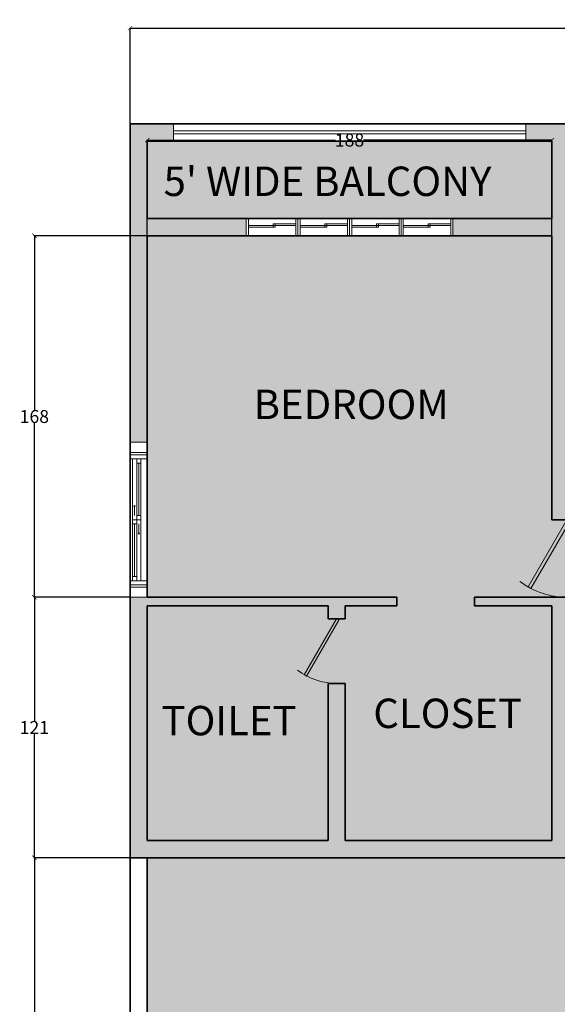
# Model space of a CAD drawing. Units: inches. Extents: x 1704 to 6393, y -157 to 1172.
# Tile 121 of 122: x 5732 to 5982, y 376 to 834. Entities that reach past the tile are written whole.
import ezdxf

# ---------------------------------------------------------------- set-up
doc = ezdxf.new("R2010")
doc.units = ezdxf.units.IN
doc.header["$MEASUREMENT"] = 0
for name, color, linetype, lineweight in [('A-ANNO-DIMS', 7, 'Continuous', 13), ('A-AREA-IDEN', 7, 'Continuous', 18), ('A-WALL-PATT', 7, 'Continuous', 13), ('DOORS', 160, 'Continuous', 18), ('GLASS PANEL FASADE', 4, 'Continuous', 18), ('WALLS', 7, 'Continuous', 35), ('WINDOWS', 2, 'Continuous', 18)]:
    doc.layers.add(name, color=color, linetype=linetype, lineweight=lineweight)
doc.layers.add('A-FLOR-PATT', color=7, linetype='Continuous', lineweight=13, true_color=0xf2f2f2)
doc.styles.get("Standard").update_dxf_attribs({"font": 'arial.ttf'})
doc.dimstyles.get("Standard").update_dxf_attribs({"dimtxt": 6, "dimasz": 2, "dimexe": 0.18, "dimexo": 0.0625, "dimgap": 0.09, "dimtad": 0, "dimtih": 1, "dimtoh": 1, "dimdec": 1, "dimzin": 0, "dimdsep": 46, "dimlunit": 3, "dimtxsty": 'Standard', "dimblk": 'ARCHTICK', "dimcen": 0.09, "dimadec": 0, "dimazin": 0, "dimtfac": 1, "dimtdec": 1, "dimtofl": 0, "dimtmove": 0, "dimatfit": 3, "dimfxl": 1, "dimtolj": 1, "dimtzin": 0, "dimarcsym": 0})

# ---------------------------------------------------------------- blocks, each defined once
blk = doc.blocks.new('Door - Left Hung 36 in.')
blk.add_lwpolyline([(0.75, -1.3), (0, 0), (31.18, 18), (31.93, 16.7)], close=True)
blk.add_arc((0, 0), 36, 0, 37.3101)
blk = doc.blocks.new('WIN-SLIDER-72')
for p, q in [((0, 72), (0, 0)), ((0, 72), (8, 72)), ((8, 66.25), (8, 72)), ((0, 67.23), (8, 67.23)), ((1.17, 36), (1.17, 64.3)), ((8, 7.7), (8, 64.3)), ((3.12, 37.95), (3.12, 62.35)), ((4.1, 37.95), (4.1, 62.35)), ((5.07, 37.95), (5.07, 62.35)), ((2.14, 37.95), (2.14, 42.14)), ((1.17, 9.65), (1.17, 34.05)), ((2.14, 9.65), (2.14, 34.05)), ((3.12, 9.65), (3.12, 34.05)), ((4.1, 34.05), (4.1, 29.86)), ((5.07, 36), (5.07, 7.7)), ((0, 4.77), (8, 4.77)), ((8, 5.75), (8, 0)), ((0, 0), (8, 0))]:
    blk.add_line(p, q)
for points in [[(8, 64.3), (8, 66.25), (0, 66.25), (0, 64.3)], [(5.07, 62.35), (5.07, 64.3), (3.12, 64.3), (3.12, 62.35)], [(2.14, 42.65), (1.85, 42.14), (2.44, 42.14)], [(5.07, 36), (5.07, 37.95), (3.12, 37.95), (3.12, 36)], [(3.12, 34.05), (3.12, 36), (1.17, 36), (1.17, 34.05)], [(4.1, 29.35), (3.8, 29.86), (4.39, 29.86)], [(3.12, 7.7), (3.12, 9.65), (1.17, 9.65), (1.17, 7.7)], [(8, 7.7), (8, 5.75), (0, 5.75), (0, 7.7)]]:
    blk.add_lwpolyline(points, close=True)
blk = doc.blocks.new('GLAZ-FOUR-PANEL-96')
for p, q in [((96, 8), (0, 8)), ((0, 8), (0, 0)), ((1, 8), (1, 0)), ((12.51, 4.77), (1, 4.77)), ((12.51, 4.77), (12.51, 5.55)), ((12.51, 5.55), (23, 5.55)), ((12.51, 4), (12.51, 4.77)), ((12.51, 4.77), (23, 4.77)), ((13.51, 4), (13.51, 5.55)), ((23, 8), (23, 0)), ((24, 8), (24, 0)), ((25, 8), (25, 0)), ((36.51, 4.77), (25, 4.77)), ((36.51, 4.77), (36.51, 5.55)), ((36.51, 5.55), (47, 5.55)), ((36.51, 4), (36.51, 4.77)), ((36.51, 4.77), (47, 4.77)), ((37.51, 4), (37.51, 5.55)), ((47, 8), (47, 0)), ((48, 8), (48, 0)), ((49, 8), (49, 0)), ((60.51, 4.77), (49, 4.77)), ((60.51, 4.77), (60.51, 5.55)), ((60.51, 5.55), (71, 5.55)), ((60.51, 4), (60.51, 4.77)), ((60.51, 4.77), (71, 4.77)), ((61.51, 4), (61.51, 5.55)), ((71, 8), (71, 0)), ((72, 8), (72, 0)), ((73, 8), (73, 0)), ((84.51, 4.77), (73, 4.77)), ((84.51, 4.77), (84.51, 5.55)), ((84.51, 5.55), (95, 5.55)), ((84.51, 4), (84.51, 4.77)), ((84.51, 4.77), (95, 4.77)), ((85.51, 4), (85.51, 5.55)), ((95, 0), (95, 8)), ((96, 0), (96, 8)), ((1, 4), (12.51, 4)), ((12.51, 4), (13.51, 4)), ((25, 4), (36.51, 4)), ((36.51, 4), (37.51, 4)), ((49, 4), (60.51, 4)), ((60.51, 4), (61.51, 4)), ((73, 4), (84.51, 4)), ((84.51, 4), (85.51, 4)), ((0, 0), (96, 0))]:
    blk.add_line(p, q)
blk = doc.blocks.new('GLAZ-PANEL-164')
for p, q in [((163.71, 4.7), (0, 4.7)), ((163.71, 3.3), (0, 3.3))]:
    blk.add_line(p, q)
blk.add_lwpolyline([(163.71, 8), (163.71, 0), (0, 0), (0, 8)], close=True)
blk = doc.blocks.new('_ArchTick')
at = {"color": 0, "linetype": 'ByBlock', "const_width": 0.15}
blk.add_lwpolyline([(-0.5, -0.5), (0.5, 0.5)], dxfattribs=at)
blk = doc.blocks.new('*D119')
at = {"layer": 'A-ANNO-DIMS', "color": 0, "lineweight": -2, "transparency": 16777216}
for p, q in [((5783.59, 785.54), (5783.59, 830.11)), ((5783.59, 829.93), (6055.87, 829.93)), ((6341.59, 829.93), (6069.31, 829.93)), ((6341.59, 644.54), (6341.59, 830.11))]:
    blk.add_line(p, q, dxfattribs=at)
at = {"layer": 'Defpoints', "color": 0, "lineweight": -3, "transparency": 16777216}
for p in [(6341.59, 829.93), (5783.59, 785.48), (6341.59, 644.48)]:
    blk.add_point(p, dxfattribs=at)
at = {"layer": 'A-ANNO-DIMS', "color": 0, "lineweight": -2, "transparency": 16777216, "xscale": 2, "yscale": 2, "zscale": 2, "rotation": 180}
blk.add_blockref('_ArchTick', (5783.59, 829.93), dxfattribs=at)
at = {"layer": 'A-ANNO-DIMS', "color": 0, "lineweight": -2, "transparency": 16777216, "xscale": 2, "yscale": 2, "zscale": 2}
blk.add_blockref('_ArchTick', (6341.59, 829.93), dxfattribs=at)
at = {"layer": 'A-ANNO-DIMS', "color": 0, "transparency": 16777216, "insert": (6062.59, 829.93), "char_height": 6, "attachment_point": 5}
blk.add_mtext('\\A1;558', dxfattribs=at)
blk = doc.blocks.new('*D123')
at = {"layer": 'A-ANNO-DIMS', "color": 0, "lineweight": -2, "transparency": 16777216}
for p, q in [((5783.53, 444.48), (5738.96, 444.48)), ((5739.14, 444.48), (5739.14, 267.63)), ((5739.14, 84.48), (5739.14, 261.32)), ((5783.54, 84.48), (5738.96, 84.48))]:
    blk.add_line(p, q, dxfattribs=at)
at = {"layer": 'Defpoints', "color": 0, "lineweight": -3, "transparency": 16777216}
for p in [(5739.14, 444.48), (5783.59, 444.48), (5783.6, 84.48)]:
    blk.add_point(p, dxfattribs=at)
at = {"layer": 'A-ANNO-DIMS', "color": 0, "lineweight": -2, "transparency": 16777216, "xscale": 2, "yscale": 2, "zscale": 2}
for p, rotation in [((5739.14, 444.48), 90), ((5739.14, 84.48), 270)]:
    blk.add_blockref('_ArchTick', p, dxfattribs=dict(at, rotation=rotation))
at = {"layer": 'A-ANNO-DIMS', "color": 0, "transparency": 16777216, "insert": (5739.14, 264.48), "char_height": 6, "attachment_point": 5}
blk.add_mtext('\\A1;360', dxfattribs=at)
blk = doc.blocks.new('*D124')
at = {"layer": 'A-ANNO-DIMS', "color": 0, "lineweight": -2, "transparency": 16777216}
for p, q in [((5783.53, 565.48), (5738.96, 565.48)), ((5739.14, 565.48), (5739.14, 508.08)), ((5739.14, 444.48), (5739.14, 501.88)), ((5783.53, 444.48), (5738.96, 444.48))]:
    blk.add_line(p, q, dxfattribs=at)
at = {"layer": 'Defpoints', "color": 0, "lineweight": -3, "transparency": 16777216}
for p in [(5739.14, 565.48), (5783.59, 565.48), (5783.59, 444.48)]:
    blk.add_point(p, dxfattribs=at)
at = {"layer": 'A-ANNO-DIMS', "color": 0, "lineweight": -2, "transparency": 16777216, "xscale": 2, "yscale": 2, "zscale": 2}
for p, rotation in [((5739.14, 565.48), 90), ((5739.14, 444.48), 270)]:
    blk.add_blockref('_ArchTick', p, dxfattribs=dict(at, rotation=rotation))
at = {"layer": 'A-ANNO-DIMS', "color": 0, "transparency": 16777216, "insert": (5739.14, 504.98), "char_height": 6, "attachment_point": 5}
blk.add_mtext('\\A1;121', dxfattribs=at)
blk = doc.blocks.new('*D125')
at = {"layer": 'A-ANNO-DIMS', "color": 0, "lineweight": -2, "transparency": 16777216}
for p, q in [((5791.53, 733.48), (5738.96, 733.48)), ((5739.14, 733.48), (5739.14, 652.63)), ((5739.14, 565.48), (5739.14, 646.32)), ((5783.53, 565.48), (5738.96, 565.48))]:
    blk.add_line(p, q, dxfattribs=at)
at = {"layer": 'Defpoints', "color": 0, "lineweight": -3, "transparency": 16777216}
for p in [(5739.14, 733.48), (5791.59, 733.48), (5783.59, 565.48)]:
    blk.add_point(p, dxfattribs=at)
at = {"layer": 'A-ANNO-DIMS', "color": 0, "lineweight": -2, "transparency": 16777216, "xscale": 2, "yscale": 2, "zscale": 2}
for p, rotation in [((5739.14, 733.48), 90), ((5739.14, 565.48), 270)]:
    blk.add_blockref('_ArchTick', p, dxfattribs=dict(at, rotation=rotation))
at = {"layer": 'A-ANNO-DIMS', "color": 0, "transparency": 16777216, "insert": (5739.14, 649.48), "char_height": 6, "attachment_point": 5}
blk.add_mtext('\\A1;168', dxfattribs=at)
blk = doc.blocks.new('*D126')
at = {"layer": 'A-ANNO-DIMS', "color": 0, "lineweight": -2, "transparency": 16777216}
for p, q in [((5791.59, 733.54), (5791.59, 778.11)), ((5791.59, 777.93), (5879.15, 777.93)), ((5979.59, 777.93), (5892.03, 777.93)), ((5979.59, 733.54), (5979.59, 778.11))]:
    blk.add_line(p, q, dxfattribs=at)
at = {"layer": 'Defpoints', "color": 0, "lineweight": -3, "transparency": 16777216}
for p in [(5979.59, 777.93), (5791.59, 733.48), (5979.59, 733.48)]:
    blk.add_point(p, dxfattribs=at)
at = {"layer": 'A-ANNO-DIMS', "color": 0, "lineweight": -2, "transparency": 16777216, "xscale": 2, "yscale": 2, "zscale": 2, "rotation": 180}
blk.add_blockref('_ArchTick', (5791.59, 777.93), dxfattribs=at)
at = {"layer": 'A-ANNO-DIMS', "color": 0, "lineweight": -2, "transparency": 16777216, "xscale": 2, "yscale": 2, "zscale": 2}
blk.add_blockref('_ArchTick', (5979.59, 777.93), dxfattribs=at)
at = {"layer": 'A-ANNO-DIMS', "color": 0, "transparency": 16777216, "insert": (5885.59, 777.93), "char_height": 6, "attachment_point": 5}
blk.add_mtext('\\A1;188', dxfattribs=at)

msp = doc.modelspace()

# ---------------------------------------------------------------- hatches: boundary and pattern name
at = {"layer": 'A-FLOR-PATT', "transparency": 33554559}
h = msp.add_hatch(color=256, dxfattribs=at)
h.dxf.hatch_style = 1
h.paths.add_polyline_path([(5979.59, 777.478), (5791.59, 777.478), (5791.59, 741.478), (5979.59, 741.478)], flags=17)
h.paths.add_polyline_path([(5979.59, 733.478), (5791.59, 733.478), (5791.59, 565.478), (5907.59, 565.478), (5907.59, 561.478), (5883.59, 561.478), (5883.59, 555.478), (5875.59, 555.478), (5875.59, 561.478), (5791.59, 561.478), (5791.59, 452.478), (5875.59, 452.478), (5875.59, 525.478), (5883.59, 525.478), (5883.59, 452.478), (5979.59, 452.478), (5979.59, 561.478), (5943.59, 561.478), (5943.59, 565.478), (5979.59, 565.478), (5987.59, 565.478), (5987.59, 444.478), (5791.59, 444.478), (5791.603, 92.478), (6059.59, 92.478), (6059.59, 292.478), (6101.682, 292.478), (6101.682, 284.478), (6067.59, 284.478), (6067.59, 164.478), (6079.59, 164.478), (6079.59, 156.478), (6067.59, 156.478), (6067.59, -11.522), (6307.59, -11.522), (6307.59, 108.478), (6307.59, 117.524), (6307.59, 156.478), (6115.59, 156.478), (6115.59, 164.478), (6307.59, 164.478), (6307.59, 236.478), (6307.59, 262.478), (6307.59, 284.478), (6137.682, 284.478), (6137.682, 292.478), (6307.59, 292.478), (6307.59, 428.478), (6068.59, 428.478), (6060.59, 428.478), (6060.59, 455.978), (6068.59, 455.978), (6068.59, 435.478), (6130.59, 435.478), (6130.59, 500.478), (6068.59, 500.478), (6068.59, 479.978), (6060.59, 479.978), (6060.59, 505.478), (6135.59, 505.478), (6135.59, 497.478), (6135.59, 436.478), (6183.59, 436.478), (6183.59, 454.978), (6187.59, 454.978), (6187.59, 436.478), (6262.788, 436.478), (6262.788, 497.478), (6187.59, 497.478), (6187.59, 478.978), (6183.59, 478.978), (6183.59, 497.478), (6159.59, 497.478), (6159.59, 505.478), (6161.98, 505.478), (6161.98, 549.478), (6137.98, 549.478), (6137.98, 555.478), (6077.98, 555.478), (6077.98, 557.478), (6077.98, 601.478), (6029.59, 601.478), (6029.59, 609.478), (6035.59, 609.478), (6207.59, 609.478), (6207.59, 641.478), (6211.59, 641.478), (6211.59, 609.478), (6223.59, 609.478), (6307.59, 609.478), (6307.59, 677.478), (6271.59, 677.478), (6271.59, 681.478), (6307.59, 681.478), (6307.59, 735.174), (6211.59, 735.174), (6211.59, 681.478), (6247.59, 681.478), (6247.59, 677.478), (6211.59, 677.478), (6207.59, 677.478), (6207.59, 777.478), (5987.59, 777.478), (5987.59, 609.478), (5993.59, 609.478), (5993.59, 601.478), (5979.59, 601.478)])
h.paths.add_polyline_path([(6307.59, 601.478), (6261.59, 601.478), (6261.59, 505.478), (6307.59, 505.478), (6307.59, 535.478)], flags=17)
h.paths.add_polyline_path([(6161.98, 601.478), (6138.98, 601.478), (6138.98, 557.478), (6161.98, 557.478)], flags=17)
h.paths.add_polyline_path([(6257.59, 601.478), (6242.98, 601.478), (6242.98, 557.478), (6257.59, 557.478)], flags=17)
h.paths.add_polyline_path([(6117.98, 601.478), (6108.98, 601.478), (6108.98, 557.478), (6117.98, 557.478)], flags=17)
h.paths.add_polyline_path([(6107.98, 601.478), (6098.98, 601.478), (6098.98, 557.478), (6107.98, 557.478)], flags=17)
h.paths.add_polyline_path([(6097.98, 601.478), (6088.98, 601.478), (6088.98, 557.478), (6097.98, 557.478)], flags=17)
h.paths.add_polyline_path([(6087.98, 601.478), (6078.98, 601.478), (6078.98, 557.478), (6087.98, 557.478)], flags=17)
h.paths.add_polyline_path([(6127.98, 601.478), (6118.98, 601.478), (6118.98, 557.478), (6127.98, 557.478)], flags=17)
h.paths.add_polyline_path([(6137.98, 601.478), (6128.98, 601.478), (6128.98, 557.478), (6137.98, 557.478)], flags=17)
h.paths.add_polyline_path([(6171.98, 601.478), (6162.98, 601.478), (6162.98, 557.478), (6171.98, 557.478)], flags=17)
h.paths.add_polyline_path([(6181.98, 601.478), (6172.98, 601.478), (6172.98, 557.478), (6181.98, 557.478)], flags=17)
h.paths.add_polyline_path([(6191.98, 601.478), (6182.98, 601.478), (6182.98, 557.478), (6191.98, 557.478)], flags=17)
h.paths.add_polyline_path([(6201.98, 601.478), (6192.98, 601.478), (6192.98, 557.478), (6201.98, 557.478)], flags=17)
h.paths.add_polyline_path([(6211.98, 601.478), (6202.98, 601.478), (6202.98, 557.478), (6211.98, 557.478)], flags=17)
h.paths.add_polyline_path([(6221.98, 601.478), (6212.98, 601.478), (6212.98, 557.478), (6221.98, 557.478)], flags=17)
h.paths.add_polyline_path([(6231.98, 601.478), (6222.98, 601.478), (6222.98, 557.478), (6231.98, 557.478)], flags=17)
h.paths.add_polyline_path([(6241.98, 601.478), (6232.98, 601.478), (6232.98, 557.478), (6241.98, 557.478)], flags=17)
h.paths.add_polyline_path([(6171.98, 549.478), (6162.98, 549.478), (6162.98, 505.478), (6171.98, 505.478)], flags=17)
h.paths.add_polyline_path([(6181.98, 549.478), (6172.98, 549.478), (6172.98, 505.478), (6181.98, 505.478)], flags=17)
h.paths.add_polyline_path([(6191.98, 549.478), (6182.98, 549.478), (6182.98, 505.478), (6191.98, 505.478)], flags=17)
h.paths.add_polyline_path([(6201.98, 549.478), (6192.98, 549.478), (6192.98, 505.478), (6201.98, 505.478)], flags=17)
h.paths.add_polyline_path([(6211.98, 549.478), (6202.98, 549.478), (6202.98, 505.478), (6211.98, 505.478)], flags=17)
h.paths.add_polyline_path([(6221.98, 549.478), (6212.98, 549.478), (6212.98, 505.478), (6221.98, 505.478)], flags=17)
h.paths.add_polyline_path([(6231.98, 549.478), (6222.98, 549.478), (6222.98, 505.478), (6231.98, 505.478)], flags=17)
h.paths.add_polyline_path([(6241.98, 549.478), (6232.98, 549.478), (6232.98, 505.478), (6241.98, 505.478)], flags=17)
h.paths.add_polyline_path([(6257.59, 549.478), (6242.98, 549.478), (6242.98, 505.478), (6257.59, 505.478)], flags=17)
at = {"layer": 'A-WALL-PATT', "transparency": 33554559}
h = msp.add_hatch(color=256, dxfattribs=at)
h.dxf.hatch_style = 1
h.paths.add_polyline_path([(5791.59, 733.478), (5837.59, 733.478), (5837.59, 741.478), (5791.59, 741.478), (5791.59, 777.478), (5803.735, 777.478), (5803.735, 785.478), (5783.59, 785.478), (5783.59, 637.478), (5791.59, 637.478)])
h.paths.add_polyline_path([(5987.59, 777.478), (5999.299, 777.478), (5999.299, 785.478), (5983.59, 785.478), (5967.445, 785.478), (5967.445, 777.478), (5979.59, 777.478), (5979.59, 741.478), (5933.59, 741.478), (5933.59, 733.478), (5979.59, 733.478), (5979.59, 601.478), (5993.59, 601.478), (5993.59, 609.478), (5987.59, 609.478)])
h = msp.add_hatch(color=256, dxfattribs=at)
h.dxf.hatch_style = 1
h.paths.add_polyline_path([(6315.59, 785.478), (6047.299, 785.478), (6047.299, 777.478), (6207.59, 777.478), (6207.59, 677.478), (6211.59, 677.478), (6247.59, 677.478), (6247.59, 681.478), (6211.59, 681.478), (6211.59, 777.478), (6307.59, 777.478), (6307.59, 744.478), (6307.59, 677.478), (6307.59, 609.478), (6211.59, 609.478), (6211.59, 641.478), (6207.59, 641.478), (6207.59, 609.478), (6035.59, 609.478), (6029.59, 609.478), (6029.59, 601.478), (6257.59, 601.478), (6257.59, 505.478), (6159.59, 505.478), (6159.59, 497.478), (6183.59, 497.478), (6183.59, 478.978), (6187.59, 478.978), (6187.59, 497.478), (6307.59, 497.478), (6307.59, 436.478), (6187.59, 436.478), (6187.59, 454.978), (6183.59, 454.978), (6183.59, 436.478), (6135.59, 436.478), (6135.59, 497.478), (6135.59, 505.478), (6060.59, 505.478), (6060.59, 479.978), (6068.59, 479.978), (6068.59, 500.478), (6130.59, 500.478), (6130.59, 435.478), (6068.59, 435.478), (6068.59, 455.978), (6060.59, 455.978), (6060.59, 428.478), (6187.59, 428.478), (6307.59, 428.478), (6307.59, 385.478), (6307.59, 363.289), (6315.59, 363.289), (6315.59, 402.478), (6315.59, 404.478), (6315.59, 456.478), (6315.59, 458.478), (6315.59, 497.478), (6315.59, 505.478), (6307.59, 505.478), (6261.59, 505.478), (6261.59, 601.478), (6307.59, 601.478), (6307.59, 535.478), (6315.59, 535.478), (6315.59, 602.478), (6315.59, 606.478), (6315.59, 642.478), (6315.59, 644.478)])
h.paths.add_polyline_path([(5791.59, 561.478), (5875.59, 561.478), (5875.59, 555.478), (5883.59, 555.478), (5883.59, 561.478), (5907.59, 561.478), (5907.59, 565.478), (5791.59, 565.478), (5783.59, 565.478), (5783.59, 444.478), (5987.59, 444.478), (5987.59, 565.478), (5979.59, 565.478), (5943.59, 565.478), (5943.59, 561.478), (5979.59, 561.478), (5979.59, 452.478), (5883.59, 452.478), (5883.59, 525.478), (5875.59, 525.478), (5875.59, 452.478), (5791.59, 452.478)])

# ---------------------------------------------------------------- linework, layer by layer
at = {"layer": 'WALLS'}
for p, q in [((6315.59, 785.478), (5783.59, 785.478)), ((5783.59, 785.478), (5783.59, 444.478)), ((5979.59, 777.478), (5791.59, 777.478)), ((5791.59, 777.478), (5791.59, 741.478)), ((5979.59, 741.478), (5979.59, 777.478)), ((5979.59, 741.478), (5791.59, 741.478)), ((5979.59, 733.478), (5791.59, 733.478)), ((5791.59, 733.478), (5791.59, 565.478)), ((5979.59, 601.478), (5979.59, 733.478)), ((5993.59, 601.478), (5979.59, 601.478)), ((5907.59, 565.478), (5791.59, 565.478)), ((5907.59, 561.478), (5907.59, 565.478)), ((5979.59, 565.478), (5943.59, 565.478)), ((5943.59, 561.478), (5943.59, 565.478)), ((5979.59, 565.478), (5987.59, 565.478)), ((5875.59, 561.478), (5791.59, 561.478)), ((5791.59, 561.478), (5791.59, 452.478)), ((5875.59, 561.478), (5875.59, 555.478)), ((5907.59, 561.478), (5883.59, 561.478)), ((5883.59, 561.478), (5883.59, 555.478)), ((5979.59, 561.478), (5943.59, 561.478)), ((5979.59, 452.478), (5979.59, 561.478)), ((5875.59, 555.478), (5883.59, 555.478)), ((5875.59, 525.478), (5875.59, 452.478)), ((5875.59, 525.478), (5883.59, 525.478)), ((5883.59, 525.478), (5883.59, 452.478)), ((5875.59, 452.478), (5791.59, 452.478)), ((5979.59, 452.478), (5883.59, 452.478)), ((5987.59, 444.478), (5783.59, 444.478)), ((5783.59, 444.478), (5783.603, 92.478)), ((5791.59, 444.478), (5791.603, 92.478))]:
    msp.add_line(p, q, dxfattribs=at)

# ---------------------------------------------------------------- block references
at = {"layer": 'DOORS', "rotation": 90}
for p, xscale, yscale, zscale in [((5986.59, 601.478), -1.00038572807606, 1.00038572807606, 1.00038572807606), ((5879.59, 555.478), -0.8333333333333172, 0.8333333333333172, 0.8333333333333172)]:
    msp.add_blockref('Door - Left Hung 36 in.', p, dxfattribs=dict(at, xscale=xscale, yscale=yscale, zscale=zscale))
at = {"layer": 'GLASS PANEL FASADE'}
for name, p in [('GLAZ-PANEL-164', (5803.735, 777.479)), ('GLAZ-FOUR-PANEL-96', (5837.591, 733.478))]:
    msp.add_blockref(name, p, dxfattribs=at)
at = {"layer": 'WINDOWS'}
msp.add_blockref('WIN-SLIDER-72', (5783.591, 565.478), dxfattribs=at)

# ---------------------------------------------------------------- texts
at = {"layer": 'A-AREA-IDEN'}
for s, p in [("5' WIDE BALCONY", (5799.199, 751.946)), ('BEDROOM', (5841.046, 648.282)), ('CLOSET', (5896.644, 504.716)), ('TOILET', (5798.258, 501.335))]:
    msp.add_text(s, height=13.6672, dxfattribs=at).set_placement(p)

# ---------------------------------------------------------------- dimensions: what is measured, and where the dimension line sits
at = {"layer": 'A-ANNO-DIMS'}
for base, p1, p2, picture, middle in [((6341.59, 829.928), (5783.59, 785.478), (6341.59, 644.478), '*D119', (6062.59, 829.928)), ((5979.59, 777.928), (5791.59, 733.478), (5979.59, 733.478), '*D126', (5885.59, 777.928))]:
    dim = msp.add_linear_dim(base=base, p1=p1, p2=p2, dimstyle='Standard', override={"dimdec": 0, "dimlfac": 1, "dimrnd": 0, "dimzin": 0, "dimdsep": 46, "dimlunit": 2}, dxfattribs=at)
    dim.commit()
    dim.dimension.update_dxf_attribs({"geometry": picture, "text_midpoint": middle})
for base, p1, p2, picture, middle in [((5739.14, 733.478), (5783.59, 565.478), (5791.59, 733.478), '*D125', (5739.14, 649.478)), ((5739.14, 565.478), (5783.59, 444.478), (5783.59, 565.478), '*D124', (5739.14, 504.978)), ((5739.14, 444.478), (5783.603, 84.478), (5783.59, 444.478), '*D123', (5739.14, 264.478))]:
    dim = msp.add_linear_dim(base=base, p1=p1, p2=p2, angle=90, dimstyle='Standard', override={"dimdec": 0, "dimlfac": 1, "dimrnd": 0, "dimzin": 0, "dimdsep": 46, "dimlunit": 2}, dxfattribs=at)
    dim.commit()
    dim.dimension.update_dxf_attribs({"geometry": picture, "text_midpoint": middle})

doc.saveas('drawing.dxf')
